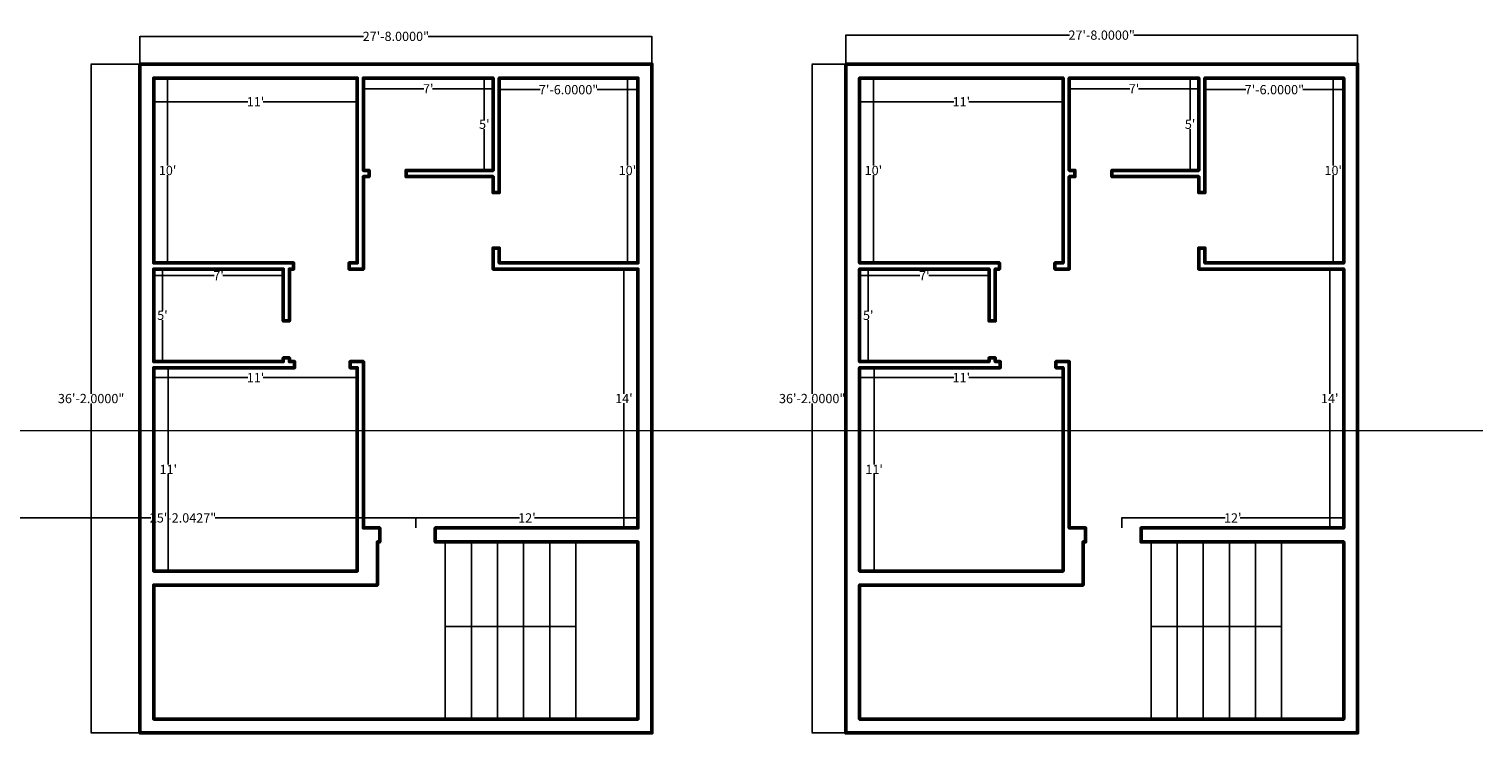
# Model space of a CAD drawing. Units: feet. Extents: x 993 to 3080, y -271 to 22562.
# Tile 4 of 4: x 1920 to 2863, y 603 to 1060. Entities that reach past the tile are written whole.
import ezdxf

# ---------------------------------------------------------------- set-up
doc = ezdxf.new("R2010")
doc.units = ezdxf.units.FT
for name, color, linetype, lineweight in [('A-ANNO-DIMS', 2, 'Continuous', 18), ('A-ANNO-SYMB', 4, 'Continuous', 18), ('A-FLOR-STRS', 3, 'Continuous', 25), ('A-WALL', 7, 'Continuous', 50)]:
    doc.layers.add(name, color=color, linetype=linetype, lineweight=lineweight)
doc.styles.get("Standard").update_dxf_attribs({"font": 'arial.ttf'})
doc.dimstyles.get("Standard").update_dxf_attribs({"dimtxt": 6, "dimasz": 0.18, "dimexe": 0.18, "dimexo": 0.0625, "dimgap": 0.09, "dimtad": 0, "dimtih": 1, "dimtoh": 1, "dimdec": 4, "dimzin": 0, "dimdsep": 46, "dimlunit": 3, "dimtxsty": 'Standard', "dimcen": 0.09, "dimadec": 0, "dimazin": 0, "dimtfac": 1, "dimtdec": 4, "dimtofl": 0, "dimtmove": 0, "dimatfit": 3, "dimfxl": 1, "dimtolj": 1, "dimtzin": 0, "dimarcsym": 0})

# ---------------------------------------------------------------- blocks, each defined once
blk = doc.blocks.new('*D17')
at = {"layer": 'A-ANNO-DIMS', "color": 0, "lineweight": -2, "transparency": 16777216}
for p, q in [((1991.96, 1037.12), (1991.96, 1055.27)), ((1992.14, 1055.09), (2137.02, 1055.09)), ((2323.78, 1055.09), (2178.89, 1055.09)), ((2323.96, 1037.12), (2323.96, 1055.27))]:
    blk.add_line(p, q, dxfattribs=at)
at = {"layer": 'A-ANNO-DIMS', "color": 0, "transparency": 16777216}
for points in [[(1992.14, 1055.12), (1992.14, 1055.06), (1991.96, 1055.09)], [(2323.78, 1055.12), (2323.78, 1055.06), (2323.96, 1055.09)]]:
    blk.add_solid(points, dxfattribs=at)
at = {"layer": 'Defpoints', "color": 0, "transparency": 16777216}
for p in [(2323.96, 1055.09), (1991.96, 1037.06), (2323.96, 1037.06)]:
    blk.add_point(p, dxfattribs=at)
at = {"layer": 'A-ANNO-DIMS', "color": 0, "transparency": 16777216, "insert": (2157.96, 1055.09), "char_height": 6, "attachment_point": 5}
blk.add_mtext('\\A1;27\'-8.0000"', dxfattribs=at)
blk = doc.blocks.new('*D18')
at = {"layer": 'A-ANNO-DIMS', "color": 0, "lineweight": -2, "transparency": 16777216}
for p, q in [((1991.9, 1037.06), (1960.17, 1037.06)), ((1960.35, 1036.88), (1960.35, 823.22)), ((1960.35, 603.24), (1960.35, 816.9)), ((1991.9, 603.06), (1960.17, 603.06))]:
    blk.add_line(p, q, dxfattribs=at)
at = {"layer": 'A-ANNO-DIMS', "color": 0, "transparency": 16777216}
for points in [[(1960.32, 1036.88), (1960.38, 1036.88), (1960.35, 1037.06)], [(1960.32, 603.24), (1960.38, 603.24), (1960.35, 603.06)]]:
    blk.add_solid(points, dxfattribs=at)
at = {"layer": 'Defpoints', "color": 0, "transparency": 16777216}
for p in [(1991.96, 1037.06), (1960.35, 603.06), (1991.96, 603.06)]:
    blk.add_point(p, dxfattribs=at)
at = {"layer": 'A-ANNO-DIMS', "color": 0, "transparency": 16777216, "insert": (1960.35, 820.06), "char_height": 6, "attachment_point": 5}
blk.add_mtext('\\A1;36\'-2.0000"', dxfattribs=at)
blk = doc.blocks.new('*D30')
at = {"layer": 'A-ANNO-DIMS', "color": 0, "lineweight": -2, "transparency": 16777216}
for p, q in [((1868.92, 736.12), (1868.92, 742.78)), ((1869.1, 742.6), (1999, 742.6)), ((2170.78, 742.6), (2040.87, 742.6)), ((2170.96, 736.12), (2170.96, 742.78))]:
    blk.add_line(p, q, dxfattribs=at)
at = {"layer": 'A-ANNO-DIMS', "color": 0, "transparency": 16777216}
for points in [[(1869.1, 742.63), (1869.1, 742.57), (1868.92, 742.6)], [(2170.78, 742.63), (2170.78, 742.57), (2170.96, 742.6)]]:
    blk.add_solid(points, dxfattribs=at)
at = {"layer": 'Defpoints', "color": 0, "transparency": 16777216}
for p in [(1868.92, 736.06), (2170.96, 742.6), (2170.96, 736.06)]:
    blk.add_point(p, dxfattribs=at)
at = {"layer": 'A-ANNO-DIMS', "color": 0, "transparency": 16777216, "insert": (2019.94, 742.6), "char_height": 6, "attachment_point": 5}
blk.add_mtext('\\A1;25\'-2.0427"', dxfattribs=at)
blk = doc.blocks.new('*D33')
at = {"layer": 'A-ANNO-DIMS', "color": 0, "lineweight": -2, "transparency": 16777216}
for p, q in [((2458.65, 1028), (2458.65, 1012.47)), ((2590.65, 1028), (2590.65, 1012.47)), ((2458.83, 1012.65), (2519.75, 1012.65)), ((2590.47, 1012.65), (2529.55, 1012.65))]:
    blk.add_line(p, q, dxfattribs=at)
at = {"layer": 'A-ANNO-DIMS', "color": 0, "transparency": 16777216}
for points in [[(2458.83, 1012.68), (2458.83, 1012.62), (2458.65, 1012.65)], [(2590.47, 1012.68), (2590.47, 1012.62), (2590.65, 1012.65)]]:
    blk.add_solid(points, dxfattribs=at)
at = {"layer": 'Defpoints', "color": 0, "transparency": 16777216}
for p in [(2458.65, 1028.06), (2590.65, 1028.06), (2590.65, 1012.65)]:
    blk.add_point(p, dxfattribs=at)
at = {"layer": 'A-ANNO-DIMS', "color": 0, "transparency": 16777216, "insert": (2524.65, 1012.65), "char_height": 6, "attachment_point": 5}
blk.add_mtext("\\A1;11'", dxfattribs=at)
blk = doc.blocks.new('*D34')
at = {"layer": 'A-ANNO-DIMS', "color": 0, "lineweight": -2, "transparency": 16777216}
for p, q in [((2458.71, 1028.06), (2467.81, 1028.06)), ((2467.63, 1027.88), (2467.63, 971.21)), ((2467.63, 908.24), (2467.63, 964.91)), ((2458.71, 908.06), (2467.81, 908.06))]:
    blk.add_line(p, q, dxfattribs=at)
at = {"layer": 'A-ANNO-DIMS', "color": 0, "transparency": 16777216}
for points in [[(2467.6, 1027.88), (2467.66, 1027.88), (2467.63, 1028.06)], [(2467.6, 908.24), (2467.66, 908.24), (2467.63, 908.06)]]:
    blk.add_solid(points, dxfattribs=at)
at = {"layer": 'Defpoints', "color": 0, "transparency": 16777216}
for p in [(2458.65, 1028.06), (2458.65, 908.06), (2467.63, 908.06)]:
    blk.add_point(p, dxfattribs=at)
at = {"layer": 'A-ANNO-DIMS', "color": 0, "transparency": 16777216, "insert": (2467.63, 968.06), "char_height": 6, "attachment_point": 5}
blk.add_mtext("\\A1;10'", dxfattribs=at)
blk = doc.blocks.new('*D35')
at = {"layer": 'A-ANNO-DIMS', "color": 0, "lineweight": -2, "transparency": 16777216}
for p, q in [((2594.65, 1028), (2594.65, 1020.88)), ((2678.65, 1028), (2678.65, 1020.88)), ((2594.83, 1021.06), (2633.82, 1021.06)), ((2678.47, 1021.06), (2639.47, 1021.06))]:
    blk.add_line(p, q, dxfattribs=at)
at = {"layer": 'A-ANNO-DIMS', "color": 0, "transparency": 16777216}
for points in [[(2594.83, 1021.09), (2594.83, 1021.03), (2594.65, 1021.06)], [(2678.47, 1021.09), (2678.47, 1021.03), (2678.65, 1021.06)]]:
    blk.add_solid(points, dxfattribs=at)
at = {"layer": 'Defpoints', "color": 0, "transparency": 16777216}
for p in [(2594.65, 1028.06), (2678.65, 1028.06), (2678.65, 1021.06)]:
    blk.add_point(p, dxfattribs=at)
at = {"layer": 'A-ANNO-DIMS', "color": 0, "transparency": 16777216, "insert": (2636.65, 1021.06), "char_height": 6, "attachment_point": 5}
blk.add_mtext("\\A1;7'", dxfattribs=at)
blk = doc.blocks.new('*D36')
at = {"layer": 'A-ANNO-DIMS', "color": 0, "lineweight": -2, "transparency": 16777216}
for p, q in [((2678.59, 1028.06), (2672.81, 1028.06)), ((2672.99, 1027.88), (2672.99, 1001.2)), ((2672.99, 968.24), (2672.99, 994.92)), ((2678.59, 968.06), (2672.81, 968.06))]:
    blk.add_line(p, q, dxfattribs=at)
at = {"layer": 'A-ANNO-DIMS', "color": 0, "transparency": 16777216}
for points in [[(2672.96, 1027.88), (2673.02, 1027.88), (2672.99, 1028.06)], [(2672.96, 968.24), (2673.02, 968.24), (2672.99, 968.06)]]:
    blk.add_solid(points, dxfattribs=at)
at = {"layer": 'Defpoints', "color": 0, "transparency": 16777216}
for p in [(2672.99, 1028.06), (2678.65, 1028.06), (2678.65, 968.06)]:
    blk.add_point(p, dxfattribs=at)
at = {"layer": 'A-ANNO-DIMS', "color": 0, "transparency": 16777216, "insert": (2672.99, 998.06), "char_height": 6, "attachment_point": 5}
blk.add_mtext("\\A1;5'", dxfattribs=at)
blk = doc.blocks.new('*D37')
at = {"layer": 'A-ANNO-DIMS', "color": 0, "lineweight": -2, "transparency": 16777216}
for p, q in [((2682.65, 1028), (2682.65, 1020.32)), ((2772.65, 1028), (2772.65, 1020.32)), ((2682.83, 1020.5), (2709.12, 1020.5)), ((2772.47, 1020.5), (2746.18, 1020.5))]:
    blk.add_line(p, q, dxfattribs=at)
at = {"layer": 'A-ANNO-DIMS', "color": 0, "transparency": 16777216}
for points in [[(2682.83, 1020.53), (2682.83, 1020.47), (2682.65, 1020.5)], [(2772.47, 1020.53), (2772.47, 1020.47), (2772.65, 1020.5)]]:
    blk.add_solid(points, dxfattribs=at)
at = {"layer": 'Defpoints', "color": 0, "transparency": 16777216}
for p in [(2682.65, 1028.06), (2772.65, 1028.06), (2682.65, 1020.5)]:
    blk.add_point(p, dxfattribs=at)
at = {"layer": 'A-ANNO-DIMS', "color": 0, "transparency": 16777216, "insert": (2727.65, 1020.5), "char_height": 6, "attachment_point": 5}
blk.add_mtext('\\A1;7\'-6.0000"', dxfattribs=at)
blk = doc.blocks.new('*D38')
at = {"layer": 'A-ANNO-DIMS', "color": 0, "lineweight": -2, "transparency": 16777216}
for p, q in [((2772.59, 1028.06), (2765.63, 1028.06)), ((2765.81, 1027.88), (2765.81, 971.21)), ((2765.81, 908.24), (2765.81, 964.91)), ((2772.59, 908.06), (2765.63, 908.06))]:
    blk.add_line(p, q, dxfattribs=at)
at = {"layer": 'A-ANNO-DIMS', "color": 0, "transparency": 16777216}
for points in [[(2765.78, 1027.88), (2765.84, 1027.88), (2765.81, 1028.06)], [(2765.78, 908.24), (2765.84, 908.24), (2765.81, 908.06)]]:
    blk.add_solid(points, dxfattribs=at)
at = {"layer": 'Defpoints', "color": 0, "transparency": 16777216}
for p in [(2772.65, 1028.06), (2765.81, 908.06), (2772.65, 908.06)]:
    blk.add_point(p, dxfattribs=at)
at = {"layer": 'A-ANNO-DIMS', "color": 0, "transparency": 16777216, "insert": (2765.81, 968.06), "char_height": 6, "attachment_point": 5}
blk.add_mtext("\\A1;10'", dxfattribs=at)
blk = doc.blocks.new('*D39')
at = {"layer": 'A-ANNO-DIMS', "color": 0, "lineweight": -2, "transparency": 16777216}
for p, q in [((2458.65, 904), (2458.65, 899.62)), ((2458.83, 899.8), (2497.82, 899.8)), ((2542.47, 899.8), (2503.47, 899.8)), ((2542.65, 904), (2542.65, 899.62))]:
    blk.add_line(p, q, dxfattribs=at)
at = {"layer": 'A-ANNO-DIMS', "color": 0, "transparency": 16777216}
for points in [[(2458.83, 899.83), (2458.83, 899.77), (2458.65, 899.8)], [(2542.47, 899.83), (2542.47, 899.77), (2542.65, 899.8)]]:
    blk.add_solid(points, dxfattribs=at)
at = {"layer": 'Defpoints', "color": 0, "transparency": 16777216}
for p in [(2458.65, 904.06), (2458.65, 899.8), (2542.65, 904.06)]:
    blk.add_point(p, dxfattribs=at)
at = {"layer": 'A-ANNO-DIMS', "color": 0, "transparency": 16777216, "insert": (2500.65, 899.8), "char_height": 6, "attachment_point": 5}
blk.add_mtext("\\A1;7'", dxfattribs=at)
blk = doc.blocks.new('*D40')
at = {"layer": 'A-ANNO-DIMS', "color": 0, "lineweight": -2, "transparency": 16777216}
for p, q in [((2458.71, 904.06), (2464.46, 904.06)), ((2464.28, 903.88), (2464.28, 877.2)), ((2464.28, 844.24), (2464.28, 870.92)), ((2458.71, 844.06), (2464.46, 844.06))]:
    blk.add_line(p, q, dxfattribs=at)
at = {"layer": 'A-ANNO-DIMS', "color": 0, "transparency": 16777216}
for points in [[(2464.25, 903.88), (2464.31, 903.88), (2464.28, 904.06)], [(2464.25, 844.24), (2464.31, 844.24), (2464.28, 844.06)]]:
    blk.add_solid(points, dxfattribs=at)
at = {"layer": 'Defpoints', "color": 0, "transparency": 16777216}
for p in [(2458.65, 904.06), (2458.65, 844.06), (2464.28, 844.06)]:
    blk.add_point(p, dxfattribs=at)
at = {"layer": 'A-ANNO-DIMS', "color": 0, "transparency": 16777216, "insert": (2464.28, 874.06), "char_height": 6, "attachment_point": 5}
blk.add_mtext("\\A1;5'", dxfattribs=at)
blk = doc.blocks.new('*D41')
at = {"layer": 'A-ANNO-DIMS', "color": 0, "lineweight": -2, "transparency": 16777216}
for p, q in [((2458.71, 840.06), (2468.27, 840.06)), ((2468.09, 839.88), (2468.09, 777.16)), ((2468.09, 708.24), (2468.09, 770.96)), ((2458.71, 708.06), (2468.27, 708.06))]:
    blk.add_line(p, q, dxfattribs=at)
at = {"layer": 'A-ANNO-DIMS', "color": 0, "transparency": 16777216}
for points in [[(2468.06, 839.88), (2468.12, 839.88), (2468.09, 840.06)], [(2468.06, 708.24), (2468.12, 708.24), (2468.09, 708.06)]]:
    blk.add_solid(points, dxfattribs=at)
at = {"layer": 'Defpoints', "color": 0, "transparency": 16777216}
for p in [(2458.65, 840.06), (2458.65, 708.06), (2468.09, 708.06)]:
    blk.add_point(p, dxfattribs=at)
at = {"layer": 'A-ANNO-DIMS', "color": 0, "transparency": 16777216, "insert": (2468.09, 774.06), "char_height": 6, "attachment_point": 5}
blk.add_mtext("\\A1;11'", dxfattribs=at)
blk = doc.blocks.new('*D42')
at = {"layer": 'A-ANNO-DIMS', "color": 0, "lineweight": -2, "transparency": 16777216}
for p, q in [((2458.65, 840), (2458.65, 833.46)), ((2590.65, 840), (2590.65, 833.46)), ((2458.83, 833.64), (2519.75, 833.64)), ((2590.47, 833.64), (2529.55, 833.64))]:
    blk.add_line(p, q, dxfattribs=at)
at = {"layer": 'A-ANNO-DIMS', "color": 0, "transparency": 16777216}
for points in [[(2458.83, 833.67), (2458.83, 833.61), (2458.65, 833.64)], [(2590.47, 833.67), (2590.47, 833.61), (2590.65, 833.64)]]:
    blk.add_solid(points, dxfattribs=at)
at = {"layer": 'Defpoints', "color": 0, "transparency": 16777216}
for p in [(2458.65, 840.06), (2590.65, 840.06), (2590.65, 833.64)]:
    blk.add_point(p, dxfattribs=at)
at = {"layer": 'A-ANNO-DIMS', "color": 0, "transparency": 16777216, "insert": (2524.65, 833.64), "char_height": 6, "attachment_point": 5}
blk.add_mtext("\\A1;11'", dxfattribs=at)
blk = doc.blocks.new('*D43')
at = {"layer": 'A-ANNO-DIMS', "color": 0, "lineweight": -2, "transparency": 16777216}
for p, q in [((2772.59, 904.06), (2763.36, 904.06)), ((2763.54, 903.88), (2763.54, 823.16)), ((2763.54, 736.24), (2763.54, 816.96)), ((2772.59, 736.06), (2763.36, 736.06))]:
    blk.add_line(p, q, dxfattribs=at)
at = {"layer": 'A-ANNO-DIMS', "color": 0, "transparency": 16777216}
for points in [[(2763.51, 903.88), (2763.57, 903.88), (2763.54, 904.06)], [(2763.51, 736.24), (2763.57, 736.24), (2763.54, 736.06)]]:
    blk.add_solid(points, dxfattribs=at)
at = {"layer": 'Defpoints', "color": 0, "transparency": 16777216}
for p in [(2772.65, 904.06), (2763.54, 736.06), (2772.65, 736.06)]:
    blk.add_point(p, dxfattribs=at)
at = {"layer": 'A-ANNO-DIMS', "color": 0, "transparency": 16777216, "insert": (2763.54, 820.06), "char_height": 6, "attachment_point": 5}
blk.add_mtext("\\A1;14'", dxfattribs=at)
blk = doc.blocks.new('*D44')
at = {"layer": 'A-ANNO-DIMS', "color": 0, "lineweight": -2, "transparency": 16777216}
for p, q in [((2628.65, 736.12), (2628.65, 742.78)), ((2628.83, 742.6), (2695.75, 742.6)), ((2772.47, 742.6), (2705.55, 742.6)), ((2772.65, 736.12), (2772.65, 742.78))]:
    blk.add_line(p, q, dxfattribs=at)
at = {"layer": 'A-ANNO-DIMS', "color": 0, "transparency": 16777216}
for points in [[(2628.83, 742.63), (2628.83, 742.57), (2628.65, 742.6)], [(2772.47, 742.63), (2772.47, 742.57), (2772.65, 742.6)]]:
    blk.add_solid(points, dxfattribs=at)
at = {"layer": 'Defpoints', "color": 0, "transparency": 16777216}
for p in [(2628.65, 742.6), (2628.65, 736.06), (2772.65, 736.06)]:
    blk.add_point(p, dxfattribs=at)
at = {"layer": 'A-ANNO-DIMS', "color": 0, "transparency": 16777216, "insert": (2700.65, 742.6), "char_height": 6, "attachment_point": 5}
blk.add_mtext("\\A1;12'", dxfattribs=at)
blk = doc.blocks.new('*D45')
at = {"layer": 'A-ANNO-DIMS', "color": 0, "lineweight": -2, "transparency": 16777216}
for p, q in [((2000.96, 1028), (2000.96, 1012.47)), ((2132.96, 1028), (2132.96, 1012.47)), ((2001.14, 1012.65), (2062.06, 1012.65)), ((2132.78, 1012.65), (2071.86, 1012.65))]:
    blk.add_line(p, q, dxfattribs=at)
at = {"layer": 'A-ANNO-DIMS', "color": 0, "transparency": 16777216}
for points in [[(2001.14, 1012.68), (2001.14, 1012.62), (2000.96, 1012.65)], [(2132.78, 1012.68), (2132.78, 1012.62), (2132.96, 1012.65)]]:
    blk.add_solid(points, dxfattribs=at)
at = {"layer": 'Defpoints', "color": 0, "transparency": 16777216}
for p in [(2000.96, 1028.06), (2132.96, 1028.06), (2132.96, 1012.65)]:
    blk.add_point(p, dxfattribs=at)
at = {"layer": 'A-ANNO-DIMS', "color": 0, "transparency": 16777216, "insert": (2066.96, 1012.65), "char_height": 6, "attachment_point": 5}
blk.add_mtext("\\A1;11'", dxfattribs=at)
blk = doc.blocks.new('*D46')
at = {"layer": 'A-ANNO-DIMS', "color": 0, "lineweight": -2, "transparency": 16777216}
for p, q in [((2001.02, 1028.06), (2010.12, 1028.06)), ((2009.94, 1027.88), (2009.94, 971.21)), ((2009.94, 908.24), (2009.94, 964.91)), ((2001.02, 908.06), (2010.12, 908.06))]:
    blk.add_line(p, q, dxfattribs=at)
at = {"layer": 'A-ANNO-DIMS', "color": 0, "transparency": 16777216}
for points in [[(2009.91, 1027.88), (2009.97, 1027.88), (2009.94, 1028.06)], [(2009.91, 908.24), (2009.97, 908.24), (2009.94, 908.06)]]:
    blk.add_solid(points, dxfattribs=at)
at = {"layer": 'Defpoints', "color": 0, "transparency": 16777216}
for p in [(2000.96, 1028.06), (2000.96, 908.06), (2009.94, 908.06)]:
    blk.add_point(p, dxfattribs=at)
at = {"layer": 'A-ANNO-DIMS', "color": 0, "transparency": 16777216, "insert": (2009.94, 968.06), "char_height": 6, "attachment_point": 5}
blk.add_mtext("\\A1;10'", dxfattribs=at)
blk = doc.blocks.new('*D47')
at = {"layer": 'A-ANNO-DIMS', "color": 0, "lineweight": -2, "transparency": 16777216}
for p, q in [((2136.96, 1028), (2136.96, 1020.88)), ((2220.96, 1028), (2220.96, 1020.88)), ((2137.14, 1021.06), (2176.13, 1021.06)), ((2220.78, 1021.06), (2181.78, 1021.06))]:
    blk.add_line(p, q, dxfattribs=at)
at = {"layer": 'A-ANNO-DIMS', "color": 0, "transparency": 16777216}
for points in [[(2137.14, 1021.09), (2137.14, 1021.03), (2136.96, 1021.06)], [(2220.78, 1021.09), (2220.78, 1021.03), (2220.96, 1021.06)]]:
    blk.add_solid(points, dxfattribs=at)
at = {"layer": 'Defpoints', "color": 0, "transparency": 16777216}
for p in [(2136.96, 1028.06), (2220.96, 1028.06), (2220.96, 1021.06)]:
    blk.add_point(p, dxfattribs=at)
at = {"layer": 'A-ANNO-DIMS', "color": 0, "transparency": 16777216, "insert": (2178.96, 1021.06), "char_height": 6, "attachment_point": 5}
blk.add_mtext("\\A1;7'", dxfattribs=at)
blk = doc.blocks.new('*D48')
at = {"layer": 'A-ANNO-DIMS', "color": 0, "lineweight": -2, "transparency": 16777216}
for p, q in [((2220.9, 1028.06), (2215.12, 1028.06)), ((2215.3, 1027.88), (2215.3, 1001.2)), ((2215.3, 968.24), (2215.3, 994.92)), ((2220.9, 968.06), (2215.12, 968.06))]:
    blk.add_line(p, q, dxfattribs=at)
at = {"layer": 'A-ANNO-DIMS', "color": 0, "transparency": 16777216}
for points in [[(2215.27, 1027.88), (2215.33, 1027.88), (2215.3, 1028.06)], [(2215.27, 968.24), (2215.33, 968.24), (2215.3, 968.06)]]:
    blk.add_solid(points, dxfattribs=at)
at = {"layer": 'Defpoints', "color": 0, "transparency": 16777216}
for p in [(2215.3, 1028.06), (2220.96, 1028.06), (2220.96, 968.06)]:
    blk.add_point(p, dxfattribs=at)
at = {"layer": 'A-ANNO-DIMS', "color": 0, "transparency": 16777216, "insert": (2215.3, 998.06), "char_height": 6, "attachment_point": 5}
blk.add_mtext("\\A1;5'", dxfattribs=at)
blk = doc.blocks.new('*D49')
at = {"layer": 'A-ANNO-DIMS', "color": 0, "lineweight": -2, "transparency": 16777216}
for p, q in [((2224.96, 1028), (2224.96, 1020.32)), ((2314.96, 1028), (2314.96, 1020.32)), ((2225.14, 1020.5), (2251.43, 1020.5)), ((2314.78, 1020.5), (2288.49, 1020.5))]:
    blk.add_line(p, q, dxfattribs=at)
at = {"layer": 'A-ANNO-DIMS', "color": 0, "transparency": 16777216}
for points in [[(2225.14, 1020.53), (2225.14, 1020.47), (2224.96, 1020.5)], [(2314.78, 1020.53), (2314.78, 1020.47), (2314.96, 1020.5)]]:
    blk.add_solid(points, dxfattribs=at)
at = {"layer": 'Defpoints', "color": 0, "transparency": 16777216}
for p in [(2224.96, 1028.06), (2314.96, 1028.06), (2224.96, 1020.5)]:
    blk.add_point(p, dxfattribs=at)
at = {"layer": 'A-ANNO-DIMS', "color": 0, "transparency": 16777216, "insert": (2269.96, 1020.5), "char_height": 6, "attachment_point": 5}
blk.add_mtext('\\A1;7\'-6.0000"', dxfattribs=at)
blk = doc.blocks.new('*D50')
at = {"layer": 'A-ANNO-DIMS', "color": 0, "lineweight": -2, "transparency": 16777216}
for p, q in [((2314.9, 1028.06), (2307.94, 1028.06)), ((2308.12, 1027.88), (2308.12, 971.21)), ((2308.12, 908.24), (2308.12, 964.91)), ((2314.9, 908.06), (2307.94, 908.06))]:
    blk.add_line(p, q, dxfattribs=at)
at = {"layer": 'A-ANNO-DIMS', "color": 0, "transparency": 16777216}
for points in [[(2308.09, 1027.88), (2308.15, 1027.88), (2308.12, 1028.06)], [(2308.09, 908.24), (2308.15, 908.24), (2308.12, 908.06)]]:
    blk.add_solid(points, dxfattribs=at)
at = {"layer": 'Defpoints', "color": 0, "transparency": 16777216}
for p in [(2314.96, 1028.06), (2308.12, 908.06), (2314.96, 908.06)]:
    blk.add_point(p, dxfattribs=at)
at = {"layer": 'A-ANNO-DIMS', "color": 0, "transparency": 16777216, "insert": (2308.12, 968.06), "char_height": 6, "attachment_point": 5}
blk.add_mtext("\\A1;10'", dxfattribs=at)
blk = doc.blocks.new('*D51')
at = {"layer": 'A-ANNO-DIMS', "color": 0, "lineweight": -2, "transparency": 16777216}
for p, q in [((2000.96, 904), (2000.96, 899.62)), ((2001.14, 899.8), (2040.13, 899.8)), ((2084.78, 899.8), (2045.78, 899.8)), ((2084.96, 904), (2084.96, 899.62))]:
    blk.add_line(p, q, dxfattribs=at)
at = {"layer": 'A-ANNO-DIMS', "color": 0, "transparency": 16777216}
for points in [[(2001.14, 899.83), (2001.14, 899.77), (2000.96, 899.8)], [(2084.78, 899.83), (2084.78, 899.77), (2084.96, 899.8)]]:
    blk.add_solid(points, dxfattribs=at)
at = {"layer": 'Defpoints', "color": 0, "transparency": 16777216}
for p in [(2000.96, 904.06), (2000.96, 899.8), (2084.96, 904.06)]:
    blk.add_point(p, dxfattribs=at)
at = {"layer": 'A-ANNO-DIMS', "color": 0, "transparency": 16777216, "insert": (2042.96, 899.8), "char_height": 6, "attachment_point": 5}
blk.add_mtext("\\A1;7'", dxfattribs=at)
blk = doc.blocks.new('*D52')
at = {"layer": 'A-ANNO-DIMS', "color": 0, "lineweight": -2, "transparency": 16777216}
for p, q in [((2001.02, 904.06), (2006.77, 904.06)), ((2006.59, 903.88), (2006.59, 877.2)), ((2006.59, 844.24), (2006.59, 870.92)), ((2001.02, 844.06), (2006.77, 844.06))]:
    blk.add_line(p, q, dxfattribs=at)
at = {"layer": 'A-ANNO-DIMS', "color": 0, "transparency": 16777216}
for points in [[(2006.56, 903.88), (2006.62, 903.88), (2006.59, 904.06)], [(2006.56, 844.24), (2006.62, 844.24), (2006.59, 844.06)]]:
    blk.add_solid(points, dxfattribs=at)
at = {"layer": 'Defpoints', "color": 0, "transparency": 16777216}
for p in [(2000.96, 904.06), (2000.96, 844.06), (2006.59, 844.06)]:
    blk.add_point(p, dxfattribs=at)
at = {"layer": 'A-ANNO-DIMS', "color": 0, "transparency": 16777216, "insert": (2006.59, 874.06), "char_height": 6, "attachment_point": 5}
blk.add_mtext("\\A1;5'", dxfattribs=at)
blk = doc.blocks.new('*D53')
at = {"layer": 'A-ANNO-DIMS', "color": 0, "lineweight": -2, "transparency": 16777216}
for p, q in [((2001.02, 840.06), (2010.58, 840.06)), ((2010.4, 839.88), (2010.4, 777.16)), ((2010.4, 708.24), (2010.4, 770.96)), ((2001.02, 708.06), (2010.58, 708.06))]:
    blk.add_line(p, q, dxfattribs=at)
at = {"layer": 'A-ANNO-DIMS', "color": 0, "transparency": 16777216}
for points in [[(2010.37, 839.88), (2010.43, 839.88), (2010.4, 840.06)], [(2010.37, 708.24), (2010.43, 708.24), (2010.4, 708.06)]]:
    blk.add_solid(points, dxfattribs=at)
at = {"layer": 'Defpoints', "color": 0, "transparency": 16777216}
for p in [(2000.96, 840.06), (2000.96, 708.06), (2010.4, 708.06)]:
    blk.add_point(p, dxfattribs=at)
at = {"layer": 'A-ANNO-DIMS', "color": 0, "transparency": 16777216, "insert": (2010.4, 774.06), "char_height": 6, "attachment_point": 5}
blk.add_mtext("\\A1;11'", dxfattribs=at)
blk = doc.blocks.new('*D54')
at = {"layer": 'A-ANNO-DIMS', "color": 0, "lineweight": -2, "transparency": 16777216}
for p, q in [((2000.96, 840), (2000.96, 833.46)), ((2132.96, 840), (2132.96, 833.46)), ((2001.14, 833.64), (2062.06, 833.64)), ((2132.78, 833.64), (2071.86, 833.64))]:
    blk.add_line(p, q, dxfattribs=at)
at = {"layer": 'A-ANNO-DIMS', "color": 0, "transparency": 16777216}
for points in [[(2001.14, 833.67), (2001.14, 833.61), (2000.96, 833.64)], [(2132.78, 833.67), (2132.78, 833.61), (2132.96, 833.64)]]:
    blk.add_solid(points, dxfattribs=at)
at = {"layer": 'Defpoints', "color": 0, "transparency": 16777216}
for p in [(2000.96, 840.06), (2132.96, 840.06), (2132.96, 833.64)]:
    blk.add_point(p, dxfattribs=at)
at = {"layer": 'A-ANNO-DIMS', "color": 0, "transparency": 16777216, "insert": (2066.96, 833.64), "char_height": 6, "attachment_point": 5}
blk.add_mtext("\\A1;11'", dxfattribs=at)
blk = doc.blocks.new('*D55')
at = {"layer": 'A-ANNO-DIMS', "color": 0, "lineweight": -2, "transparency": 16777216}
for p, q in [((2314.9, 904.06), (2305.67, 904.06)), ((2305.85, 903.88), (2305.85, 823.16)), ((2305.85, 736.24), (2305.85, 816.96)), ((2314.9, 736.06), (2305.67, 736.06))]:
    blk.add_line(p, q, dxfattribs=at)
at = {"layer": 'A-ANNO-DIMS', "color": 0, "transparency": 16777216}
for points in [[(2305.82, 903.88), (2305.88, 903.88), (2305.85, 904.06)], [(2305.82, 736.24), (2305.88, 736.24), (2305.85, 736.06)]]:
    blk.add_solid(points, dxfattribs=at)
at = {"layer": 'Defpoints', "color": 0, "transparency": 16777216}
for p in [(2314.96, 904.06), (2305.85, 736.06), (2314.96, 736.06)]:
    blk.add_point(p, dxfattribs=at)
at = {"layer": 'A-ANNO-DIMS', "color": 0, "transparency": 16777216, "insert": (2305.85, 820.06), "char_height": 6, "attachment_point": 5}
blk.add_mtext("\\A1;14'", dxfattribs=at)
blk = doc.blocks.new('*D56')
at = {"layer": 'A-ANNO-DIMS', "color": 0, "lineweight": -2, "transparency": 16777216}
for p, q in [((2170.96, 736.12), (2170.96, 742.78)), ((2171.14, 742.6), (2238.06, 742.6)), ((2314.78, 742.6), (2247.86, 742.6)), ((2314.96, 736.12), (2314.96, 742.78))]:
    blk.add_line(p, q, dxfattribs=at)
at = {"layer": 'A-ANNO-DIMS', "color": 0, "transparency": 16777216}
for points in [[(2171.14, 742.63), (2171.14, 742.57), (2170.96, 742.6)], [(2314.78, 742.63), (2314.78, 742.57), (2314.96, 742.6)]]:
    blk.add_solid(points, dxfattribs=at)
at = {"layer": 'Defpoints', "color": 0, "transparency": 16777216}
for p in [(2170.96, 742.6), (2170.96, 736.06), (2314.96, 736.06)]:
    blk.add_point(p, dxfattribs=at)
at = {"layer": 'A-ANNO-DIMS', "color": 0, "transparency": 16777216, "insert": (2242.96, 742.6), "char_height": 6, "attachment_point": 5}
blk.add_mtext("\\A1;12'", dxfattribs=at)
blk = doc.blocks.new('*D57')
at = {"layer": 'A-ANNO-DIMS', "color": 0, "lineweight": -2, "transparency": 16777216}
for p, q in [((2449.65, 1037.12), (2449.65, 1056.07)), ((2781.65, 1037.12), (2781.65, 1056.07)), ((2449.83, 1055.89), (2594.71, 1055.89)), ((2781.47, 1055.89), (2636.58, 1055.89))]:
    blk.add_line(p, q, dxfattribs=at)
at = {"layer": 'A-ANNO-DIMS', "color": 0, "transparency": 16777216}
for points in [[(2449.83, 1055.92), (2449.83, 1055.86), (2449.65, 1055.89)], [(2781.47, 1055.92), (2781.47, 1055.86), (2781.65, 1055.89)]]:
    blk.add_solid(points, dxfattribs=at)
at = {"layer": 'Defpoints', "color": 0, "transparency": 16777216}
for p in [(2781.65, 1055.89), (2449.65, 1037.06), (2781.65, 1037.06)]:
    blk.add_point(p, dxfattribs=at)
at = {"layer": 'A-ANNO-DIMS', "color": 0, "transparency": 16777216, "insert": (2615.65, 1055.89), "char_height": 6, "attachment_point": 5}
blk.add_mtext('\\A1;27\'-8.0000"', dxfattribs=at)
blk = doc.blocks.new('*D58')
at = {"layer": 'A-ANNO-DIMS', "color": 0, "lineweight": -2, "transparency": 16777216}
for p, q in [((2449.59, 1037.06), (2427.75, 1037.06)), ((2427.93, 1036.88), (2427.93, 823.22)), ((2427.93, 603.24), (2427.93, 816.9)), ((2449.59, 603.06), (2427.75, 603.06))]:
    blk.add_line(p, q, dxfattribs=at)
at = {"layer": 'A-ANNO-DIMS', "color": 0, "transparency": 16777216}
for points in [[(2427.9, 1036.88), (2427.96, 1036.88), (2427.93, 1037.06)], [(2427.9, 603.24), (2427.96, 603.24), (2427.93, 603.06)]]:
    blk.add_solid(points, dxfattribs=at)
at = {"layer": 'Defpoints', "color": 0, "transparency": 16777216}
for p in [(2449.65, 1037.06), (2427.93, 603.06), (2449.65, 603.06)]:
    blk.add_point(p, dxfattribs=at)
at = {"layer": 'A-ANNO-DIMS', "color": 0, "transparency": 16777216, "insert": (2427.93, 820.06), "char_height": 6, "attachment_point": 5}
blk.add_mtext('\\A1;36\'-2.0000"', dxfattribs=at)

msp = doc.modelspace()

# ---------------------------------------------------------------- linework, layer by layer
at = {"layer": 'A-ANNO-SYMB'}
msp.add_line((1484.89473, 799.38224), (2862.87672, 799.38224), dxfattribs=at)
at = {"layer": 'A-FLOR-STRS'}
for p, q in [((2189.95777, 727.05993), (2189.95777, 612.05993)), ((2189.95777, 612.05993), (2189.95777, 727.05993)), ((2206.90066, 727.05993), (2206.90066, 612.05993)), ((2223.84354, 727.05993), (2223.84354, 612.05993)), ((2240.78642, 727.05993), (2240.78642, 612.05993)), ((2257.7293, 727.05993), (2257.7293, 612.05993)), ((2274.67218, 727.05993), (2274.67218, 612.05993)), ((2647.64789, 612.05993), (2647.64789, 727.05993)), ((2647.64789, 727.05993), (2647.64789, 612.05993)), ((2664.59077, 727.05993), (2664.59077, 612.05993)), ((2681.53365, 727.05993), (2681.53365, 612.05993)), ((2698.47654, 727.05993), (2698.47654, 612.05993)), ((2715.41942, 727.05993), (2715.41942, 612.05993)), ((2732.3623, 727.05993), (2732.3623, 612.05993)), ((2189.95777, 672.05993), (2274.67218, 672.05993)), ((2647.64789, 672.05993), (2732.3623, 672.05993))]:
    msp.add_line(p, q, dxfattribs=at)
at = {"layer": 'A-FLOR-STRS', "extrusion": (0, -1, 0)}
for p, q in [((2274.67218, 612.05993), (2274.67218, 727.05993)), ((2732.3623, 612.05993), (2732.3623, 727.05993))]:
    msp.add_line(p, q, dxfattribs=at)
at = {"layer": 'A-FLOR-STRS'}
for points in [[(2189.95777, 612.05993, 0), (2314.95777, 612.05993, 0), (2274.67218, 612.05993, 0)], [(2647.64789, 612.05993, 0), (2772.64789, 612.05993, 0), (2732.3623, 612.05993, 0)]]:
    msp.add_polyline3d(points, dxfattribs=at)
at = {"layer": 'A-WALL'}
for points in [[(1991.95777, 1037.05993), (2323.95777, 1037.05993), (2323.95777, 603.05993), (1991.95777, 603.05993)], [(2449.64789, 1037.05993), (2781.64789, 1037.05993), (2781.64789, 603.05993), (2449.64789, 603.05993)]]:
    msp.add_lwpolyline(points, close=True, dxfattribs=at)
for points in [[(2084.95777, 844.05993), (2000.95777, 844.05993), (2000.95777, 904.05993), (2084.95777, 904.05993), (2084.95777, 870.45617), (2088.95777, 870.45617), (2088.95777, 904.05993), (2091.60171, 904.05993), (2091.60171, 908.05993), (2000.95777, 908.05993), (2000.95777, 1028.05993), (2132.95777, 1028.05993), (2132.95777, 908.05993), (2127.60171, 908.05993), (2127.60171, 904.05993), (2136.95777, 904.05993), (2136.95777, 964.05993), (2140.60941, 964.05993), (2140.60941, 968.05993), (2136.95777, 968.05993), (2136.95777, 1028.05993), (2220.95777, 1028.05993), (2220.95777, 968.05993), (2164.60941, 968.05993), (2164.60941, 964.05993), (2220.95777, 964.05993), (2220.95777, 953.73085), (2224.95777, 953.73085), (2224.95777, 1028.05993), (2314.95777, 1028.05993), (2314.95777, 908.05993), (2224.95777, 908.05993), (2224.95777, 917.73085), (2220.95777, 917.73085), (2220.95777, 904.05993), (2314.95777, 904.05993), (2314.95777, 736.05993), (2183.52843, 736.05993), (2183.52843, 727.05993), (2314.95777, 727.05993), (2314.95777, 612.05993), (2000.95777, 612.05993), (2000.95777, 699.05993), (2145.95777, 699.05993), (2145.95777, 727.05993), (2147.52843, 727.05993), (2147.52843, 736.05993), (2136.95777, 736.05993), (2136.95777, 844.05993), (2128.2338, 844.05993), (2128.2338, 840.05993), (2132.95777, 840.05993), (2132.95777, 708.05993), (2000.95777, 708.05993), (2000.95777, 840.05993), (2092.2338, 840.05993), (2092.2338, 844.05993), (2088.95777, 844.05993), (2088.95777, 846.45617), (2084.95777, 846.45617), (2084.95777, 844.05993), (2000.95777, 844.05993)], [(2542.64789, 844.05993), (2458.64789, 844.05993), (2458.64789, 904.05993), (2542.64789, 904.05993), (2542.64789, 870.45617), (2546.64789, 870.45617), (2546.64789, 904.05993), (2549.29183, 904.05993), (2549.29183, 908.05993), (2458.64789, 908.05993), (2458.64789, 1028.05993), (2590.64789, 1028.05993), (2590.64789, 908.05993), (2585.29183, 908.05993), (2585.29183, 904.05993), (2594.64789, 904.05993), (2594.64789, 964.05993), (2598.29953, 964.05993), (2598.29953, 968.05993), (2594.64789, 968.05993), (2594.64789, 1028.05993), (2678.64789, 1028.05993), (2678.64789, 968.05993), (2622.29953, 968.05993), (2622.29953, 964.05993), (2678.64789, 964.05993), (2678.64789, 953.73085), (2682.64789, 953.73085), (2682.64789, 1028.05993), (2772.64789, 1028.05993), (2772.64789, 908.05993), (2682.64789, 908.05993), (2682.64789, 917.73085), (2678.64789, 917.73085), (2678.64789, 904.05993), (2772.64789, 904.05993), (2772.64789, 736.05993), (2641.21855, 736.05993), (2641.21855, 727.05993), (2772.64789, 727.05993), (2772.64789, 612.05993), (2458.64789, 612.05993), (2458.64789, 699.05993), (2603.64789, 699.05993), (2603.64789, 727.05993), (2605.21855, 727.05993), (2605.21855, 736.05993), (2594.64789, 736.05993), (2594.64789, 844.05993), (2585.92392, 844.05993), (2585.92392, 840.05993), (2590.64789, 840.05993), (2590.64789, 708.05993), (2458.64789, 708.05993), (2458.64789, 840.05993), (2549.92392, 840.05993), (2549.92392, 844.05993), (2546.64789, 844.05993), (2546.64789, 846.45617), (2542.64789, 846.45617), (2542.64789, 844.05993), (2458.64789, 844.05993)]]:
    msp.add_lwpolyline(points, dxfattribs=at)

# ---------------------------------------------------------------- dimensions: what is measured, and where the dimension line sits
at = {"layer": 'A-ANNO-DIMS'}
for base, p1, p2, picture, middle in [((2323.95777, 1055.0926), (1991.95777, 1037.05993), (2323.95777, 1037.05993), '*D17', (2157.95777, 1055.0926)), ((2781.64789, 1055.89086), (2449.64789, 1037.05993), (2781.64789, 1037.05993), '*D57', (2615.64789, 1055.89086)), ((2132.95777, 1012.65309), (2000.95777, 1028.05993), (2132.95777, 1028.05993), '*D45', (2066.95777, 1012.65309)), ((2220.95777, 1021.06127), (2136.95777, 1028.05993), (2220.95777, 1028.05993), '*D47', (2178.95777, 1021.06127)), ((2224.95777, 1020.49688), (2314.95777, 1028.05993), (2224.95777, 1028.05993), '*D49', (2269.95777, 1020.49688)), ((2590.64789, 1012.65309), (2458.64789, 1028.05993), (2590.64789, 1028.05993), '*D33', (2524.64789, 1012.65309)), ((2678.64789, 1021.06127), (2594.64789, 1028.05993), (2678.64789, 1028.05993), '*D35', (2636.64789, 1021.06127)), ((2682.64789, 1020.49688), (2772.64789, 1028.05993), (2682.64789, 1028.05993), '*D37', (2727.64789, 1020.49688)), ((2000.95777, 899.80123), (2084.95777, 904.05993), (2000.95777, 904.05993), '*D51', (2042.95777, 899.80123)), ((2458.64789, 899.80123), (2542.64789, 904.05993), (2458.64789, 904.05993), '*D39', (2500.64789, 899.80123)), ((2132.95777, 833.63877), (2000.95777, 840.05993), (2132.95777, 840.05993), '*D54', (2066.95777, 833.63877)), ((2590.64789, 833.63877), (2458.64789, 840.05993), (2590.64789, 840.05993), '*D42', (2524.64789, 833.63877)), ((2170.95777, 742.60107), (1868.91505, 736.05993), (2170.95777, 736.05993), '*D30', (2019.93641, 742.60107)), ((2170.95777, 742.60107), (2314.95777, 736.05993), (2170.95777, 736.05993), '*D56', (2242.95777, 742.60107)), ((2628.64789, 742.60107), (2772.64789, 736.05993), (2628.64789, 736.05993), '*D44', (2700.64789, 742.60107))]:
    dim = msp.add_linear_dim(base=base, p1=p1, p2=p2, dimstyle='Standard', override={"dimclrd": 0, "dimclre": 0, "dimclrt": 0}, dxfattribs=at)
    dim.commit()
    dim.dimension.update_dxf_attribs({"geometry": picture, "text_midpoint": middle})
for base, p1, p2, picture, middle in [((1960.34667, 603.05993), (1991.95777, 1037.05993), (1991.95777, 603.05993), '*D18', (1960.34667, 820.05993)), ((2427.92839, 603.05993), (2449.64789, 1037.05993), (2449.64789, 603.05993), '*D58', (2427.92839, 820.05993)), ((2009.94401, 908.05993), (2000.95777, 1028.05993), (2000.95777, 908.05993), '*D46', (2009.94401, 968.05993)), ((2215.30015, 1028.05993), (2220.95777, 968.05993), (2220.95777, 1028.05993), '*D48', (2215.30015, 998.05993)), ((2308.12403, 908.05993), (2314.95777, 1028.05993), (2314.95777, 908.05993), '*D50', (2308.12403, 968.05993)), ((2467.63413, 908.05993), (2458.64789, 1028.05993), (2458.64789, 908.05993), '*D34', (2467.63413, 968.05993)), ((2672.99027, 1028.05993), (2678.64789, 968.05993), (2678.64789, 1028.05993), '*D36', (2672.99027, 998.05993)), ((2765.81415, 908.05993), (2772.64789, 1028.05993), (2772.64789, 908.05993), '*D38', (2765.81415, 968.05993)), ((2006.59323, 844.05993), (2000.95777, 904.05993), (2000.95777, 844.05993), '*D52', (2006.59323, 874.05993)), ((2305.85294, 736.05993), (2314.95777, 904.05993), (2314.95777, 736.05993), '*D55', (2305.85294, 820.05993)), ((2464.28335, 844.05993), (2458.64789, 904.05993), (2458.64789, 844.05993), '*D40', (2464.28335, 874.05993)), ((2763.54306, 736.05993), (2772.64789, 904.05993), (2772.64789, 736.05993), '*D43', (2763.54306, 820.05993)), ((2010.39921, 708.05993), (2000.95777, 840.05993), (2000.95777, 708.05993), '*D53', (2010.39921, 774.05993)), ((2468.08933, 708.05993), (2458.64789, 840.05993), (2458.64789, 708.05993), '*D41', (2468.08933, 774.05993))]:
    dim = msp.add_linear_dim(base=base, p1=p1, p2=p2, angle=90, dimstyle='Standard', override={"dimclrd": 0, "dimclre": 0, "dimclrt": 0}, dxfattribs=at)
    dim.commit()
    dim.dimension.update_dxf_attribs({"geometry": picture, "text_midpoint": middle})

doc.saveas('drawing.dxf')
